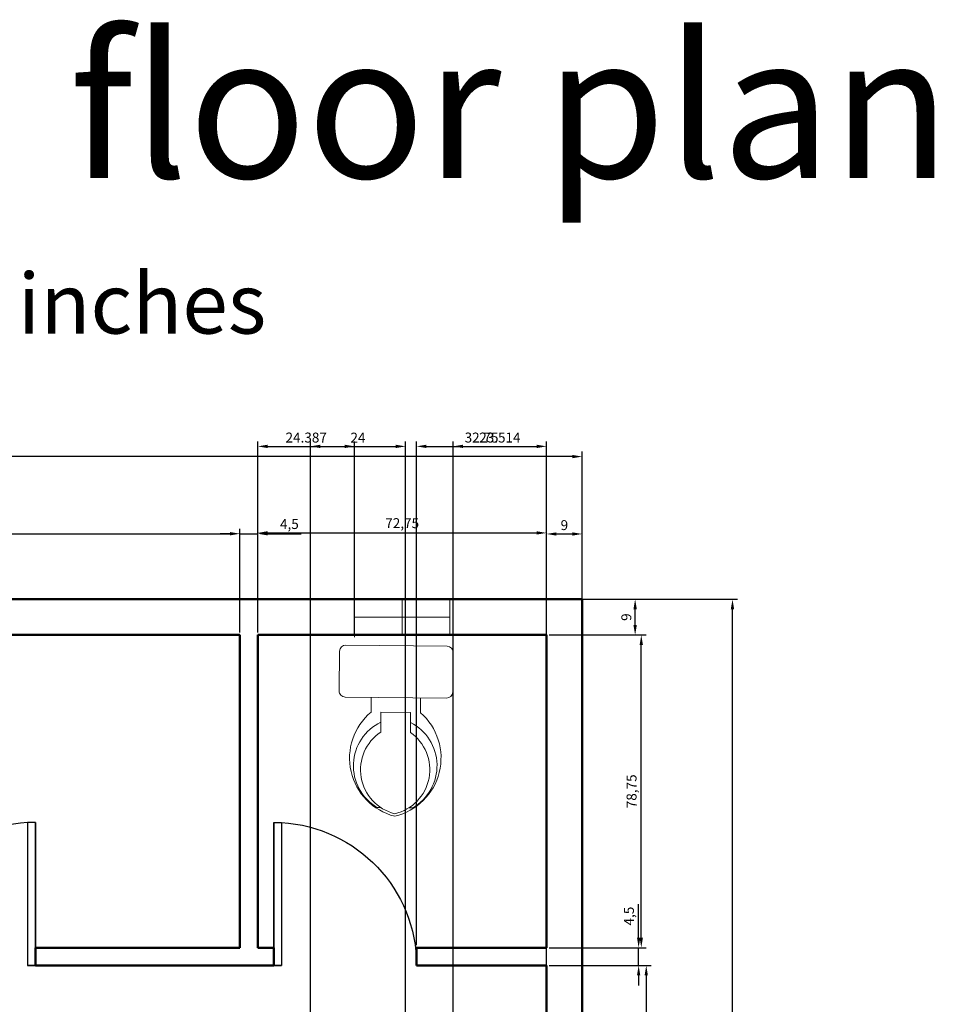
# Model space of a CAD drawing. Units: inches. Extents: x 907 to 2409, y 377 to 1163.
# Tile 8 of 9: x 1197 to 1427, y 915 to 1163. Entities that reach past the tile are written whole.
import ezdxf

# ---------------------------------------------------------------- set-up
doc = ezdxf.new("R2010")
doc.units = ezdxf.units.IN
for name, color, linetype, lineweight in [('A-ANNO-DIMS', 2, 'Continuous', 18), ('A-ANNO-TEXT', 7, 'Continuous', 25), ('A-DOOR', 3, 'Continuous', 25), ('A-FLOR-FIXT', 9, 'Continuous', 18), ('A-GLAZ', 4, 'Continuous', 18), ('A-WALL', 7, 'Continuous', 50)]:
    doc.layers.add(name, color=color, linetype=linetype, lineweight=lineweight)
doc.styles.get("Standard").update_dxf_attribs({"font": 'arial.ttf'})
doc.dimstyles.new('ISO-25', dxfattribs={"dimtxt": 2.5, "dimasz": 2.5, "dimexe": 1.25, "dimexo": 0.625, "dimtad": 1, "dimtxsty": 'Standard', "dimcen": 2.5, "dimadec": 0, "dimazin": 0, "dimtfac": 1, "dimtmove": 0, "dimatfit": 3, "dimfxl": 1, "dimarcsym": 0})

# ---------------------------------------------------------------- blocks, each defined once
blk = doc.blocks.new('A$C02F3725D')
for p, q in [((0.025, 0.69), (0.435, 0.69)), ((0, 0.505), (0, 0.665)), ((0.46, 0.665), (0.46, 0.505)), ((0.435, 0.48), (0.025, 0.48)), ((0.13, 0.48), (0.13, 0.42)), ((0.33, 0.42), (0.33, 0.48)), ((0.17, 0.34), (0.17, 0.42)), ((0.17, 0.42), (0.29, 0.42)), ((0.29, 0.34), (0.29, 0.42)), ((0.1578, 0.035), (0.1724, 0.035)), ((0.2876, 0.035), (0.3022, 0.035))]:
    blk.add_line(p, q)
for centre, radius, start, end in [((0.025, 0.665), 0.025, 90, 180), ((0.435, 0.665), 0.025, 0, 90), ((0.025, 0.505), 0.025, 180, 270), ((0.435, 0.505), 0.025, 270, 0), ((0.2874, 0.2356), 0.2425, 130.4885, 256.2965), ((0.1726, 0.2356), 0.2425, 283.7035, 49.5115), ((0.2568, 0.2042), 0.196, 116.2742, 239.6668), ((0.2032, 0.2042), 0.196, 300.3332, 63.7258), ((0.2732, 0.1883), 0.1834, 124.2157, 256.394), ((0.1868, 0.1883), 0.1834, 283.606, 55.7843)]:
    blk.add_arc(centre, radius, start, end)
blk = doc.blocks.new('*D8')
at = {"layer": 'A-ANNO-DIMS', "color": 0, "lineweight": -2, "transparency": 16777216}
for p, q in [((1064.86, 1008.5), (1064.86, 1034.62)), ((1252.36, 1008.5), (1252.36, 1034.62)), ((1067.36, 1033.37), (1249.86, 1033.37))]:
    blk.add_line(p, q, dxfattribs=at)
at = {"layer": 'A-ANNO-DIMS', "color": 0, "transparency": 16777216}
for points in [[(1067.36, 1033.79), (1067.36, 1032.95), (1064.86, 1033.37)], [(1249.86, 1033.79), (1249.86, 1032.95), (1252.36, 1033.37)]]:
    blk.add_solid(points, dxfattribs=at)
at = {"layer": 'Defpoints', "color": 0, "transparency": 16777216}
for p in [(1252.36, 1033.37), (1064.86, 1007.87), (1252.36, 1007.87)]:
    blk.add_point(p, dxfattribs=at)
at = {"layer": 'A-ANNO-DIMS', "color": 0, "transparency": 16777216, "insert": (1158.61, 1035.5), "char_height": 2.5, "attachment_point": 5}
blk.add_mtext('187,5', dxfattribs=at)
blk = doc.blocks.new('*D9')
at = {"layer": 'A-ANNO-DIMS', "color": 0, "lineweight": -2, "transparency": 16777216}
for p, q in [((1252.36, 1008.5), (1252.36, 1034.62)), ((1256.86, 1008.5), (1256.86, 1034.62)), ((1249.86, 1033.37), (1247.36, 1033.37)), ((1252.36, 1033.37), (1256.86, 1033.37)), ((1259.36, 1033.37), (1267.78, 1033.37))]:
    blk.add_line(p, q, dxfattribs=at)
at = {"layer": 'A-ANNO-DIMS', "color": 0, "transparency": 16777216}
for points in [[(1249.86, 1033.79), (1249.86, 1032.95), (1252.36, 1033.37)], [(1259.36, 1033.79), (1259.36, 1032.95), (1256.86, 1033.37)]]:
    blk.add_solid(points, dxfattribs=at)
at = {"layer": 'Defpoints', "color": 0, "transparency": 16777216}
for p in [(1256.86, 1033.37), (1252.36, 1007.87), (1256.86, 1007.87)]:
    blk.add_point(p, dxfattribs=at)
at = {"layer": 'A-ANNO-DIMS', "color": 0, "transparency": 16777216, "insert": (1264.82, 1035.49), "char_height": 2.5, "attachment_point": 5}
blk.add_mtext('4,5', dxfattribs=at)
blk = doc.blocks.new('*D10')
at = {"layer": 'A-ANNO-DIMS', "color": 0, "lineweight": -2, "transparency": 16777216}
for p, q in [((1256.86, 1008.5), (1256.86, 1034.83)), ((1329.61, 1008.5), (1329.61, 1034.83)), ((1259.36, 1033.58), (1327.11, 1033.58))]:
    blk.add_line(p, q, dxfattribs=at)
at = {"layer": 'A-ANNO-DIMS', "color": 0, "transparency": 16777216}
for points in [[(1259.36, 1034), (1259.36, 1033.16), (1256.86, 1033.58)], [(1327.11, 1034), (1327.11, 1033.16), (1329.61, 1033.58)]]:
    blk.add_solid(points, dxfattribs=at)
at = {"layer": 'Defpoints', "color": 0, "transparency": 16777216}
for p in [(1329.61, 1033.58), (1256.86, 1007.87), (1329.61, 1007.87)]:
    blk.add_point(p, dxfattribs=at)
at = {"layer": 'A-ANNO-DIMS', "color": 0, "transparency": 16777216, "insert": (1293.24, 1035.71), "char_height": 2.5, "attachment_point": 5}
blk.add_mtext('72,75', dxfattribs=at)
blk = doc.blocks.new('*D11')
at = {"layer": 'A-ANNO-DIMS', "color": 0, "lineweight": -2, "transparency": 16777216}
for p, q in [((1329.61, 1008.5), (1329.61, 1034.56)), ((1338.61, 1008.5), (1338.61, 1034.56)), ((1332.11, 1033.31), (1336.11, 1033.31))]:
    blk.add_line(p, q, dxfattribs=at)
at = {"layer": 'A-ANNO-DIMS', "color": 0, "transparency": 16777216}
for points in [[(1332.11, 1033.72), (1332.11, 1032.89), (1329.61, 1033.31)], [(1336.11, 1033.72), (1336.11, 1032.89), (1338.61, 1033.31)]]:
    blk.add_solid(points, dxfattribs=at)
at = {"layer": 'Defpoints', "color": 0, "transparency": 16777216}
for p in [(1338.61, 1033.31), (1329.61, 1007.87), (1338.61, 1007.87)]:
    blk.add_point(p, dxfattribs=at)
at = {"layer": 'A-ANNO-DIMS', "color": 0, "transparency": 16777216, "insert": (1334.11, 1035.21), "char_height": 2.5, "attachment_point": 5}
blk.add_mtext('9', dxfattribs=at)
blk = doc.blocks.new('*D12')
at = {"layer": 'A-ANNO-DIMS', "color": 0, "lineweight": -2, "transparency": 16777216}
for p, q in [((978.61, 1017.5), (978.61, 1054.05)), ((1338.61, 1017.5), (1338.61, 1054.05)), ((1336.11, 1052.8), (981.11, 1052.8))]:
    blk.add_line(p, q, dxfattribs=at)
at = {"layer": 'A-ANNO-DIMS', "color": 0, "transparency": 16777216}
for points in [[(981.11, 1053.22), (981.11, 1052.39), (978.61, 1052.8)], [(1336.11, 1053.22), (1336.11, 1052.39), (1338.61, 1052.8)]]:
    blk.add_solid(points, dxfattribs=at)
at = {"layer": 'Defpoints', "color": 0, "transparency": 16777216}
for p in [(978.61, 1052.8), (978.61, 1016.87), (1338.61, 1016.87)]:
    blk.add_point(p, dxfattribs=at)
at = {"layer": 'A-ANNO-DIMS', "color": 0, "transparency": 16777216, "insert": (1158.61, 1054.71), "char_height": 2.5, "attachment_point": 5}
blk.add_mtext('360', dxfattribs=at)
blk = doc.blocks.new('*D13')
at = {"layer": 'A-ANNO-DIMS', "color": 0, "lineweight": -2, "transparency": 16777216}
for p, q in [((1330.24, 1016.87), (1353.19, 1016.87)), ((1351.94, 1010.37), (1351.94, 1014.37)), ((1330.24, 1007.87), (1353.19, 1007.87))]:
    blk.add_line(p, q, dxfattribs=at)
at = {"layer": 'A-ANNO-DIMS', "color": 0, "transparency": 16777216}
for points in [[(1351.52, 1014.37), (1352.36, 1014.37), (1351.94, 1016.87)], [(1351.52, 1010.37), (1352.36, 1010.37), (1351.94, 1007.87)]]:
    blk.add_solid(points, dxfattribs=at)
at = {"layer": 'Defpoints', "color": 0, "transparency": 16777216}
for p in [(1329.61, 1016.87), (1351.94, 1016.87), (1329.61, 1007.87)]:
    blk.add_point(p, dxfattribs=at)
at = {"layer": 'A-ANNO-DIMS', "color": 0, "transparency": 16777216, "insert": (1350.04, 1012.37), "char_height": 2.5, "attachment_point": 5, "rotation": 90}
blk.add_mtext('9', dxfattribs=at)
blk = doc.blocks.new('*D14')
at = {"layer": 'A-ANNO-DIMS', "color": 0, "lineweight": -2, "transparency": 16777216}
for p, q in [((1330.24, 1007.87), (1354.74, 1007.87)), ((1353.49, 931.62), (1353.49, 1005.37)), ((1330.24, 929.12), (1354.74, 929.12))]:
    blk.add_line(p, q, dxfattribs=at)
at = {"layer": 'A-ANNO-DIMS', "color": 0, "transparency": 16777216}
for points in [[(1353.07, 1005.37), (1353.9, 1005.37), (1353.49, 1007.87)], [(1353.07, 931.62), (1353.9, 931.62), (1353.49, 929.12)]]:
    blk.add_solid(points, dxfattribs=at)
at = {"layer": 'Defpoints', "color": 0, "transparency": 16777216}
for p in [(1329.61, 1007.87), (1353.49, 1007.87), (1329.61, 929.12)]:
    blk.add_point(p, dxfattribs=at)
at = {"layer": 'A-ANNO-DIMS', "color": 0, "transparency": 16777216, "insert": (1351.36, 968.5), "char_height": 2.5, "attachment_point": 5, "rotation": 90}
blk.add_mtext('78,75', dxfattribs=at)
blk = doc.blocks.new('*D15')
at = {"layer": 'A-ANNO-DIMS', "color": 0, "lineweight": -2, "transparency": 16777216}
for p, q in [((1352.82, 931.62), (1352.82, 940.04)), ((1330.24, 929.12), (1354.07, 929.12)), ((1352.82, 924.62), (1352.82, 929.12)), ((1330.24, 924.62), (1354.07, 924.62)), ((1352.82, 922.12), (1352.82, 919.62))]:
    blk.add_line(p, q, dxfattribs=at)
at = {"layer": 'A-ANNO-DIMS', "color": 0, "transparency": 16777216}
for points in [[(1352.41, 931.62), (1353.24, 931.62), (1352.82, 929.12)], [(1352.41, 922.12), (1353.24, 922.12), (1352.82, 924.62)]]:
    blk.add_solid(points, dxfattribs=at)
at = {"layer": 'Defpoints', "color": 0, "transparency": 16777216}
for p in [(1329.61, 929.12), (1352.82, 929.12), (1329.61, 924.62)]:
    blk.add_point(p, dxfattribs=at)
at = {"layer": 'A-ANNO-DIMS', "color": 0, "transparency": 16777216, "insert": (1350.7, 937.08), "char_height": 2.5, "attachment_point": 5, "rotation": 90}
blk.add_mtext('4,5', dxfattribs=at)
blk = doc.blocks.new('*D16')
at = {"layer": 'A-ANNO-DIMS', "color": 0, "lineweight": -2, "transparency": 16777216}
for p, q in [((1330.24, 924.62), (1355.99, 924.62)), ((1354.74, 922.12), (1354.74, 875.37)), ((1330.24, 872.87), (1355.99, 872.87))]:
    blk.add_line(p, q, dxfattribs=at)
at = {"layer": 'A-ANNO-DIMS', "color": 0, "transparency": 16777216}
for points in [[(1354.32, 922.12), (1355.16, 922.12), (1354.74, 924.62)], [(1354.32, 875.37), (1355.16, 875.37), (1354.74, 872.87)]]:
    blk.add_solid(points, dxfattribs=at)
at = {"layer": 'Defpoints', "color": 0, "transparency": 16777216}
for p in [(1329.61, 924.62), (1329.61, 872.87), (1354.74, 872.87)]:
    blk.add_point(p, dxfattribs=at)
at = {"layer": 'A-ANNO-DIMS', "color": 0, "transparency": 16777216, "insert": (1352.61, 898.75), "char_height": 2.5, "attachment_point": 5, "rotation": 90}
blk.add_mtext('51,75', dxfattribs=at)
blk = doc.blocks.new('*D20')
at = {"layer": 'A-ANNO-DIMS', "color": 0, "lineweight": -2, "transparency": 16777216}
for p, q in [((1339.24, 1016.87), (1377.72, 1016.87)), ((1376.47, 419.37), (1376.47, 1014.37)), ((1339.24, 416.87), (1377.72, 416.87))]:
    blk.add_line(p, q, dxfattribs=at)
at = {"layer": 'A-ANNO-DIMS', "color": 0, "transparency": 16777216}
for points in [[(1376.05, 1014.37), (1376.88, 1014.37), (1376.47, 1016.87)], [(1376.05, 419.37), (1376.88, 419.37), (1376.47, 416.87)]]:
    blk.add_solid(points, dxfattribs=at)
at = {"layer": 'Defpoints', "color": 0, "transparency": 16777216}
for p in [(1338.61, 1016.87), (1376.47, 1016.87), (1338.61, 416.87)]:
    blk.add_point(p, dxfattribs=at)
at = {"layer": 'A-ANNO-DIMS', "color": 0, "transparency": 16777216, "insert": (1374.56, 716.87), "char_height": 2.5, "attachment_point": 5, "rotation": 90}
blk.add_mtext('600', dxfattribs=at)
blk = doc.blocks.new('DOOR-36IN')
for p, q in [((36, 36), (36, 0)), ((36, 0), (34, 0)), ((36, 0), (34, 0))]:
    blk.add_line(p, q)
blk.add_lwpolyline([(36, 36), (34, 36), (34, 0), (36, 0)], close=True)
blk.add_arc((36.06, 0), 36.06, 93.2732, 180)
blk = doc.blocks.new('WIN-24IN')
for p, q in [((0.53, 23.99), (0, 23.99)), ((9.53, 24), (0.53, 24)), ((5.03, 0), (5.03, 24)), ((9.53, 12), (0.53, 12)), ((9.53, 0), (0.53, 0))]:
    blk.add_line(p, q)
blk = doc.blocks.new('*D68')
at = {"layer": 'A-ANNO-DIMS', "color": 0, "lineweight": -2, "transparency": 16777216}
for p, q in [((1296.86, 929.75), (1296.86, 1056.62)), ((1329.61, 929.75), (1329.61, 1056.62)), ((1299.36, 1055.37), (1327.11, 1055.37))]:
    blk.add_line(p, q, dxfattribs=at)
at = {"layer": 'A-ANNO-DIMS', "color": 0, "transparency": 16777216}
for points in [[(1299.36, 1055.79), (1299.36, 1054.95), (1296.86, 1055.37)], [(1327.11, 1055.79), (1327.11, 1054.95), (1329.61, 1055.37)]]:
    blk.add_solid(points, dxfattribs=at)
at = {"layer": 'Defpoints', "color": 0, "transparency": 16777216}
for p in [(1329.61, 1055.37), (1296.86, 929.12), (1329.61, 929.12)]:
    blk.add_point(p, dxfattribs=at)
at = {"layer": 'A-ANNO-DIMS', "color": 0, "transparency": 16777216, "insert": (1313.24, 1057.27), "char_height": 2.5, "attachment_point": 5}
blk.add_mtext('32.75', dxfattribs=at)
blk = doc.blocks.new('*D69')
at = {"layer": 'A-ANNO-DIMS', "color": 0, "lineweight": -2, "transparency": 16777216}
for p, q in [((1256.86, 1008.5), (1256.86, 1056.62)), ((1281.25, 1007.97), (1281.25, 1056.62)), ((1259.36, 1055.37), (1278.75, 1055.37))]:
    blk.add_line(p, q, dxfattribs=at)
at = {"layer": 'A-ANNO-DIMS', "color": 0, "transparency": 16777216}
for points in [[(1259.36, 1055.79), (1259.36, 1054.95), (1256.86, 1055.37)], [(1278.75, 1055.79), (1278.75, 1054.95), (1281.25, 1055.37)]]:
    blk.add_solid(points, dxfattribs=at)
at = {"layer": 'Defpoints', "color": 0, "transparency": 16777216}
for p in [(1281.25, 1055.37), (1256.86, 1007.87), (1281.25, 1007.34)]:
    blk.add_point(p, dxfattribs=at)
at = {"layer": 'A-ANNO-DIMS', "color": 0, "transparency": 16777216, "insert": (1269.06, 1057.27), "char_height": 2.5, "attachment_point": 5}
blk.add_mtext('24.387', dxfattribs=at)
blk = doc.blocks.new('*D77')
at = {"layer": 'A-ANNO-DIMS', "color": 0, "lineweight": -2, "transparency": 16777216}
for p, q in [((1270.1, 534.51), (1270.1, 1056.62)), ((1294.1, 534.51), (1294.1, 1056.62)), ((1272.6, 1055.37), (1291.6, 1055.37))]:
    blk.add_line(p, q, dxfattribs=at)
at = {"layer": 'A-ANNO-DIMS', "color": 0, "transparency": 16777216}
for points in [[(1272.6, 1055.79), (1272.6, 1054.95), (1270.1, 1055.37)], [(1291.6, 1055.79), (1291.6, 1054.95), (1294.1, 1055.37)]]:
    blk.add_solid(points, dxfattribs=at)
at = {"layer": 'Defpoints', "color": 0, "transparency": 16777216}
for p in [(1294.1, 1055.37), (1270.1, 533.88), (1294.1, 533.88)]:
    blk.add_point(p, dxfattribs=at)
at = {"layer": 'A-ANNO-DIMS', "color": 0, "transparency": 16777216, "insert": (1282.1, 1057.25), "char_height": 2.5, "attachment_point": 5}
blk.add_mtext('24', dxfattribs=at)
blk = doc.blocks.new('*D78')
at = {"layer": 'A-ANNO-DIMS', "color": 0, "lineweight": -2, "transparency": 16777216}
for p, q in [((1306.1, 534.51), (1306.1, 1056.62)), ((1329.61, 534.51), (1329.61, 1056.62)), ((1308.6, 1055.37), (1327.11, 1055.37))]:
    blk.add_line(p, q, dxfattribs=at)
at = {"layer": 'A-ANNO-DIMS', "color": 0, "transparency": 16777216}
for points in [[(1308.6, 1055.79), (1308.6, 1054.95), (1306.1, 1055.37)], [(1327.11, 1055.79), (1327.11, 1054.95), (1329.61, 1055.37)]]:
    blk.add_solid(points, dxfattribs=at)
at = {"layer": 'Defpoints', "color": 0, "transparency": 16777216}
for p in [(1329.61, 1055.37), (1306.1, 533.88), (1329.61, 533.88)]:
    blk.add_point(p, dxfattribs=at)
at = {"layer": 'A-ANNO-DIMS', "color": 0, "transparency": 16777216, "insert": (1317.86, 1057.27), "char_height": 2.5, "attachment_point": 5}
blk.add_mtext('23.514', dxfattribs=at)

msp = doc.modelspace()

# ---------------------------------------------------------------- linework, layer by layer
at = {"layer": 'A-WALL'}
for p, q in [((978.6122, 1016.8705), (1338.6122, 1016.8705)), ((978.6122, 1016.8705), (1338.6122, 1016.8705)), ((1338.6122, 416.8705), (1338.6122, 1016.8705)), ((1338.6122, 1016.8705), (1338.6122, 926.8705)), ((1338.6122, 416.8705), (1338.6122, 1016.8705)), ((1064.8622, 1007.8705), (1252.3622, 1007.8705)), ((1064.8622, 1007.8705), (1252.3622, 1007.8705)), ((1252.3622, 1007.8705), (1252.3622, 929.1205)), ((1256.8622, 1007.8705), (1256.8622, 929.1205)), ((1256.8622, 1007.8705), (1329.6122, 1007.8705)), ((1256.8622, 1007.8705), (1329.6122, 1007.8705)), ((1329.6122, 929.1205), (1329.6122, 1007.8705)), ((1200.8622, 924.6205), (1200.8622, 929.1205)), ((1200.8622, 929.1205), (1252.3622, 929.1205)), ((1256.8622, 929.1205), (1260.8622, 929.1205)), ((1260.8622, 929.1205), (1260.8622, 924.6205)), ((1296.8622, 929.1205), (1296.8622, 924.6205)), ((1296.8622, 929.1205), (1329.6122, 929.1205)), ((1200.8622, 924.6205), (1260.8622, 924.6205)), ((1296.8622, 924.6205), (1329.6122, 924.6205)), ((1329.6122, 773.1205), (1329.6122, 924.6205))]:
    msp.add_line(p, q, dxfattribs=at)
msp.add_lwpolyline([(1216.3622, 416.8705), (1338.6122, 416.8705), (1338.6122, 1016.8705), (978.6122, 1016.8705), (978.6122, 416.8705), (1100.8622, 416.8705)], dxfattribs=at)

# ---------------------------------------------------------------- block references
at = {"layer": 'A-DOOR'}
msp.add_blockref('DOOR-36IN', (1164.8622, 924.6205), dxfattribs=at)
at = {"layer": 'A-DOOR', "extrusion": (0, 0, -1), "zscale": -1}
msp.add_blockref('DOOR-36IN', (-1296.8622, 924.6205), dxfattribs=at)
at = {"layer": 'A-FLOR-FIXT', "xscale": 62.2489048765839, "yscale": 62.2489048765839, "zscale": 62.2489048765839, "rotation": 359.4045355129811}
msp.add_blockref('A$C02F3725D', (1277.0401, 962.3763), dxfattribs=at)
at = {"layer": 'A-GLAZ', "rotation": 90.00000000000063}
msp.add_blockref('WIN-24IN', (1305.2368, 1007.3413), dxfattribs=at)

# ---------------------------------------------------------------- texts
at = {"layer": 'A-ANNO-TEXT', "attachment_point": 1}
for s, width, gutter_width, insert, char_height in [('3bhk ground floor plan', 591.346782, 180.477, (905.2958, 1159.0854), 36.095399), ('all dimensions are in inches', 399.634663, 75.8973, (992.819, 1098.9518), 15.179467)]:
    msp.add_mtext_dynamic_manual_height_columns(s, width=width, gutter_width=gutter_width, heights=[0], dxfattribs=dict(at, insert=insert, char_height=char_height))

# ---------------------------------------------------------------- dimensions: what is measured, and where the dimension line sits
at = {"layer": 'A-ANNO-DIMS'}
for base, p1, p2, override, picture, middle in [((1281.2489, 1055.3705), (1256.8622, 1007.8705), (1281.2489, 1007.3413), {"dimdec": 3, "dimlfac": 1, "dimrnd": 0, "dimzin": 0, "dimdsep": 46, "dimlunit": 2}, '*D69', (1269.0556, 1057.2728)), ((1294.0979, 1055.3705), (1270.0979, 533.8833), (1294.0979, 533.8833), {"dimdec": 0, "dimlfac": 1, "dimrnd": 0, "dimzin": 0, "dimdsep": 46, "dimlunit": 2}, '*D77', (1282.0979, 1057.2507)), ((1329.6122, 1055.3705), (1296.8622, 929.1205), (1329.6122, 929.1205), {"dimdec": 2, "dimlfac": 1, "dimrnd": 0, "dimzin": 0, "dimdsep": 46, "dimlunit": 2}, '*D68', (1313.2372, 1057.2728)), ((1329.6122, 1055.3705), (1306.0979, 533.8833), (1329.6122, 533.8833), {"dimdec": 3, "dimlfac": 1, "dimrnd": 0, "dimzin": 0, "dimdsep": 46, "dimlunit": 2}, '*D78', (1317.8551, 1057.2728)), ((978.6122, 1052.8035), (1338.6122, 1016.8705), (978.6122, 1016.8705), {"dimclrd": 0, "dimclre": 0, "dimclrt": 0}, '*D12', (1158.6122, 1054.7058)), ((1252.3622, 1033.3713), (1064.8622, 1007.8705), (1252.3622, 1007.8705), {"dimclrd": 0, "dimclre": 0, "dimclrt": 0}, '*D8', (1158.6122, 1035.4987)), ((1256.8622, 1033.3713), (1252.3622, 1007.8705), (1256.8622, 1007.8705), {"dimclrd": 0, "dimclre": 0, "dimclrt": 0}, '*D9', (1264.8227, 1035.4936)), ((1329.6122, 1033.5796), (1256.8622, 1007.8705), (1329.6122, 1007.8705), {"dimclrd": 0, "dimclre": 0, "dimclrt": 0}, '*D10', (1293.2372, 1035.707)), ((1338.6122, 1033.3056), (1329.6122, 1007.8705), (1338.6122, 1007.8705), {"dimclrd": 0, "dimclre": 0, "dimclrt": 0}, '*D11', (1334.1122, 1035.2071))]:
    dim = msp.add_linear_dim(base=base, p1=p1, p2=p2, dimstyle='ISO-25', override=override, dxfattribs=at)
    dim.commit()
    dim.dimension.update_dxf_attribs({"geometry": picture, "text_midpoint": middle})
for base, p1, p2, picture, middle in [((1351.9411, 1016.8705), (1329.6122, 1007.8705), (1329.6122, 1016.8705), '*D13', (1350.0397, 1012.3705)), ((1376.4651, 1016.8705), (1338.6122, 416.8705), (1338.6122, 1016.8705), '*D20', (1374.5637, 716.8705)), ((1353.4855, 1007.8705), (1329.6122, 929.1205), (1329.6122, 1007.8705), '*D14', (1351.3581, 968.4955)), ((1352.8217, 929.1205), (1329.6122, 924.6205), (1329.6122, 929.1205), '*D15', (1350.6995, 937.081)), ((1354.7405, 872.8705), (1329.6122, 924.6205), (1329.6122, 872.8705), '*D16', (1352.6131, 898.7455))]:
    dim = msp.add_linear_dim(base=base, p1=p1, p2=p2, angle=90, dimstyle='ISO-25', override={"dimclrd": 0, "dimclre": 0, "dimclrt": 0}, dxfattribs=at)
    dim.commit()
    dim.dimension.update_dxf_attribs({"geometry": picture, "text_midpoint": middle})

doc.saveas('drawing.dxf')
